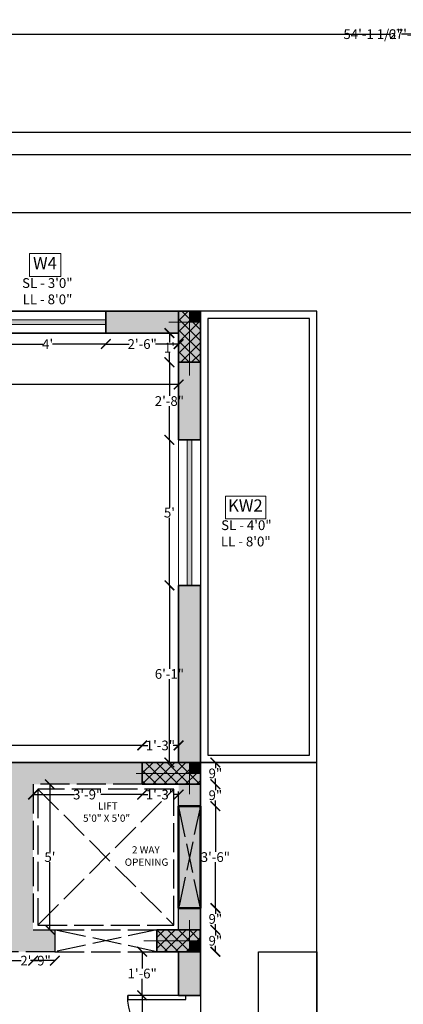
# Model space of a CAD drawing. Units: inches. Extents: x 2 to 905, y 9 to 678.
# Tile 6 of 8: x 295 to 454, y 272 to 678. Entities that reach past the tile are written whole.
import ezdxf

# ---------------------------------------------------------------- set-up
doc = ezdxf.new("R2010")
doc.units = ezdxf.units.IN
doc.linetypes.add('ACAD_ISO02W100', pattern=[15, 12, -3])
for name, color, linetype, lineweight in [('A-ANNO-DIMS', 7, 'Continuous', 18), ('A-COLS', 1, 'Continuous', 35), ('A-COLS-MARK', 1, 'Continuous', 18), ('A-COLS-MARK-PATT', 3, 'Continuous', 13), ('A-COLS-PATT', 1, 'Continuous', 13), ('A-DOOR', 7, 'Continuous', 25), ('A-FLOR', 7, 'Continuous', 25), ('A-GLAZ', 4, 'Continuous', 18), ('A-GLAZ-PATT', 4, 'Continuous', 13), ('A-TRAN', 1, 'Continuous', 50), ('A-TRAN-HIDN', 7, 'ACAD_ISO02W100', 25), ('A-WALL', 7, 'Continuous', 35), ('C-PROP', 7, 'Continuous', 25)]:
    doc.layers.add(name, color=color, linetype=linetype, lineweight=lineweight)
for name, color, linetype, lineweight, true_color in [('A-ANNO-IDEN', 251, 'Continuous', 18, 0x636466), ('A-ANNO-TEXT', 251, 'Continuous', 18, 0x636466), ('A-AREA-IDEN', 252, 'Continuous', 18, 0x989898), ('A-WALL-PATT', 252, 'Continuous', 13, 0x939598)]:
    doc.layers.add(name, color=color, linetype=linetype, lineweight=lineweight, true_color=true_color)
doc.styles.add('PDF ArialMT', font='arial.ttf')
doc.styles.add('PDF Century Gothic Bold', font='txt')
doc.styles.get("Standard").update_dxf_attribs({"font": 'arial.ttf'})
doc.dimstyles.get("Standard").update_dxf_attribs({"dimtxt": 4, "dimasz": 4, "dimexe": 0.18, "dimexo": 0.0625, "dimgap": 0.09, "dimtad": 0, "dimtih": 1, "dimtoh": 1, "dimdec": 1, "dimzin": 0, "dimdsep": 46, "dimlunit": 3, "dimtxsty": 'Standard', "dimblk": 'ARCHTICK', "dimcen": 0, "dimse1": 1, "dimse2": 1, "dimclrt": 1, "dimadec": 0, "dimazin": 0, "dimtfac": 1, "dimtdec": 1, "dimtofl": 0, "dimtmove": 0, "dimatfit": 3, "dimfxl": 1, "dimtolj": 1, "dimtzin": 0, "dimarcsym": 0})

# ---------------------------------------------------------------- blocks, each defined once
blk = doc.blocks.new('*U2')
for p, q in [((0, 0), (0, -6)), ((24, 0), (24, -6))]:
    blk.add_line(p, q)
blk.add_lwpolyline([(0, 0), (0, 24), (1.75, 24), (1.75, 0)], close=True)
blk.add_arc((0, 0), 24, 0, 90)
blk = doc.blocks.new('_ArchTick')
at = {"color": 0, "linetype": 'ByBlock', "const_width": 0.15}
blk.add_lwpolyline([(-0.5, -0.5), (0.5, 0.5)], dxfattribs=at)
blk = doc.blocks.new('*D11')
at = {"layer": 'A-ANNO-DIMS', "color": 0, "lineweight": -2, "transparency": 16777216}
for p, q in [((218.07, 548.58), (218.07, 462.21)), ((218.07, 371.58), (218.07, 457.95))]:
    blk.add_line(p, q, dxfattribs=at)
at = {"layer": 'Defpoints', "color": 0, "transparency": 16777216}
for p in [(360.93, 548.58), (218.07, 371.58), (360.93, 371.58)]:
    blk.add_point(p, dxfattribs=at)
at = {"layer": 'A-ANNO-DIMS', "color": 0, "lineweight": -2, "transparency": 16777216, "xscale": 4, "yscale": 4, "zscale": 4}
for p, rotation in [((218.07, 548.58), 90), ((218.07, 371.58), 270)]:
    blk.add_blockref('_ArchTick', p, dxfattribs=dict(at, rotation=rotation))
at = {"layer": 'A-ANNO-DIMS', "color": 0, "transparency": 16777216, "insert": (218.07, 460.08), "char_height": 4, "attachment_point": 5}
blk.add_mtext('\\A1;14\'-9"', dxfattribs=at)
blk = doc.blocks.new('*D12')
at = {"layer": 'A-ANNO-DIMS', "color": 0, "lineweight": -2, "transparency": 16777216}
for p, q in [((125.43, 527.38), (234.08, 527.38)), ((360.93, 527.38), (252.29, 527.38))]:
    blk.add_line(p, q, dxfattribs=at)
at = {"layer": 'Defpoints', "color": 0, "transparency": 16777216}
for p in [(125.43, 548.58), (360.93, 548.58), (360.93, 527.38)]:
    blk.add_point(p, dxfattribs=at)
at = {"layer": 'A-ANNO-DIMS', "color": 0, "lineweight": -2, "transparency": 16777216, "xscale": 4, "yscale": 4, "zscale": 4, "rotation": 180}
blk.add_blockref('_ArchTick', (125.43, 527.38), dxfattribs=at)
at = {"layer": 'A-ANNO-DIMS', "color": 0, "lineweight": -2, "transparency": 16777216, "xscale": 4, "yscale": 4, "zscale": 4}
blk.add_blockref('_ArchTick', (360.93, 527.38), dxfattribs=at)
at = {"layer": 'A-ANNO-DIMS', "color": 0, "transparency": 16777216, "insert": (243.18, 527.38), "char_height": 4, "attachment_point": 5}
blk.add_mtext('\\A1;19\'-7.5"', dxfattribs=at)
blk = doc.blocks.new('*D21')
at = {"layer": 'A-ANNO-DIMS', "color": 0, "lineweight": -2, "transparency": 16777216}
for p, q in [((345.92, 275.58), (345.92, 253.67)), ((345.92, 227.58), (345.92, 249.49))]:
    blk.add_line(p, q, dxfattribs=at)
at = {"layer": 'Defpoints', "color": 0, "transparency": 16777216}
for p in [(345.92, 275.58), (360.93, 275.58), (351.93, 227.58)]:
    blk.add_point(p, dxfattribs=at)
at = {"layer": 'A-ANNO-DIMS', "color": 0, "lineweight": -2, "transparency": 16777216, "xscale": 4, "yscale": 4, "zscale": 4}
for p, rotation in [((345.92, 275.58), 90), ((345.92, 227.58), 270)]:
    blk.add_blockref('_ArchTick', p, dxfattribs=dict(at, rotation=rotation))
at = {"layer": 'A-ANNO-DIMS', "color": 0, "transparency": 16777216, "insert": (345.92, 251.58), "char_height": 4, "attachment_point": 5}
blk.add_mtext("\\A1;4'", dxfattribs=at)
blk = doc.blocks.new('*D22')
at = {"layer": 'A-ANNO-DIMS', "color": 0, "lineweight": -2, "transparency": 16777216}
for p, q in [((345.92, 293.58), (345.92, 286.71)), ((345.92, 275.58), (345.92, 282.45))]:
    blk.add_line(p, q, dxfattribs=at)
at = {"layer": 'Defpoints', "color": 0, "transparency": 16777216}
for p in [(345.92, 293.58), (360.93, 293.58), (360.93, 275.58)]:
    blk.add_point(p, dxfattribs=at)
at = {"layer": 'A-ANNO-DIMS', "color": 0, "lineweight": -2, "transparency": 16777216, "xscale": 4, "yscale": 4, "zscale": 4}
for p, rotation in [((345.92, 293.58), 90), ((345.92, 275.58), 270)]:
    blk.add_blockref('_ArchTick', p, dxfattribs=dict(at, rotation=rotation))
at = {"layer": 'A-ANNO-DIMS', "color": 0, "transparency": 16777216, "insert": (345.92, 284.58), "char_height": 4, "attachment_point": 5}
blk.add_mtext('\\A1;1\'-6"', dxfattribs=at)
blk = doc.blocks.new('*D30')
at = {"layer": 'A-ANNO-DIMS', "color": 0, "lineweight": -2, "transparency": 16777216}
for p, q in [((285.93, 289.89), (295.97, 289.89)), ((309.93, 289.89), (299.9, 289.89))]:
    blk.add_line(p, q, dxfattribs=at)
at = {"layer": 'Defpoints', "color": 0, "transparency": 16777216}
for p in [(285.93, 293.58), (309.93, 293.58), (309.93, 289.89)]:
    blk.add_point(p, dxfattribs=at)
at = {"layer": 'A-ANNO-DIMS', "color": 0, "lineweight": -2, "transparency": 16777216, "xscale": 4, "yscale": 4, "zscale": 4, "rotation": 180}
blk.add_blockref('_ArchTick', (285.93, 289.89), dxfattribs=at)
at = {"layer": 'A-ANNO-DIMS', "color": 0, "lineweight": -2, "transparency": 16777216, "xscale": 4, "yscale": 4, "zscale": 4}
blk.add_blockref('_ArchTick', (309.93, 289.89), dxfattribs=at)
at = {"layer": 'A-ANNO-DIMS', "color": 0, "transparency": 16777216, "insert": (297.93, 289.89), "char_height": 4, "attachment_point": 5}
blk.add_mtext("\\A1;2'", dxfattribs=at)
blk = doc.blocks.new('*D31')
at = {"layer": 'A-ANNO-DIMS', "color": 0, "lineweight": -2, "transparency": 16777216}
for p, q in [((300.93, 289.89), (303.04, 289.89)), ((309.93, 289.89), (307.82, 289.89))]:
    blk.add_line(p, q, dxfattribs=at)
at = {"layer": 'Defpoints', "color": 0, "transparency": 16777216}
for p in [(300.93, 302.58), (309.93, 293.58), (300.93, 289.89)]:
    blk.add_point(p, dxfattribs=at)
at = {"layer": 'A-ANNO-DIMS', "color": 0, "lineweight": -2, "transparency": 16777216, "xscale": 4, "yscale": 4, "zscale": 4, "rotation": 180}
blk.add_blockref('_ArchTick', (300.93, 289.89), dxfattribs=at)
at = {"layer": 'A-ANNO-DIMS', "color": 0, "lineweight": -2, "transparency": 16777216, "xscale": 4, "yscale": 4, "zscale": 4}
blk.add_blockref('_ArchTick', (309.93, 289.89), dxfattribs=at)
at = {"layer": 'A-ANNO-DIMS', "color": 0, "transparency": 16777216, "insert": (305.43, 289.89), "char_height": 4, "attachment_point": 5}
blk.add_mtext('\\A1;9"', dxfattribs=at)
blk = doc.blocks.new('*D41')
at = {"layer": 'A-ANNO-DIMS', "color": 0, "lineweight": -2, "transparency": 16777216}
for p, q in [((300.93, 358.35), (318.03, 358.35)), ((345.93, 358.35), (328.84, 358.35))]:
    blk.add_line(p, q, dxfattribs=at)
at = {"layer": 'Defpoints', "color": 0, "transparency": 16777216}
for p in [(300.93, 362.58), (345.93, 362.58), (345.93, 358.35)]:
    blk.add_point(p, dxfattribs=at)
at = {"layer": 'A-ANNO-DIMS', "color": 0, "lineweight": -2, "transparency": 16777216, "xscale": 4, "yscale": 4, "zscale": 4, "rotation": 180}
blk.add_blockref('_ArchTick', (300.93, 358.35), dxfattribs=at)
at = {"layer": 'A-ANNO-DIMS', "color": 0, "lineweight": -2, "transparency": 16777216, "xscale": 4, "yscale": 4, "zscale": 4}
blk.add_blockref('_ArchTick', (345.93, 358.35), dxfattribs=at)
at = {"layer": 'A-ANNO-DIMS', "color": 0, "transparency": 16777216, "insert": (323.43, 358.35), "char_height": 4, "attachment_point": 5}
blk.add_mtext('\\A1;3\'-9"', dxfattribs=at)
blk = doc.blocks.new('*D42')
at = {"layer": 'A-ANNO-DIMS', "color": 0, "lineweight": -2, "transparency": 16777216}
for p, q in [((345.93, 358.35), (348.22, 358.35)), ((360.93, 358.35), (358.65, 358.35))]:
    blk.add_line(p, q, dxfattribs=at)
at = {"layer": 'Defpoints', "color": 0, "transparency": 16777216}
for p in [(345.93, 362.58), (360.93, 362.58), (360.93, 358.35)]:
    blk.add_point(p, dxfattribs=at)
at = {"layer": 'A-ANNO-DIMS', "color": 0, "lineweight": -2, "transparency": 16777216, "xscale": 4, "yscale": 4, "zscale": 4, "rotation": 180}
blk.add_blockref('_ArchTick', (345.93, 358.35), dxfattribs=at)
at = {"layer": 'A-ANNO-DIMS', "color": 0, "lineweight": -2, "transparency": 16777216, "xscale": 4, "yscale": 4, "zscale": 4}
blk.add_blockref('_ArchTick', (360.93, 358.35), dxfattribs=at)
at = {"layer": 'A-ANNO-DIMS', "color": 0, "transparency": 16777216, "insert": (353.43, 358.35), "char_height": 4, "attachment_point": 5}
blk.add_mtext('\\A1;1\'-3"', dxfattribs=at)
blk = doc.blocks.new('*D43')
at = {"layer": 'A-ANNO-DIMS', "color": 0, "lineweight": -2, "transparency": 16777216}
for p, q in [((307.87, 362.58), (307.87, 334.7)), ((307.87, 302.58), (307.87, 330.45))]:
    blk.add_line(p, q, dxfattribs=at)
at = {"layer": 'Defpoints', "color": 0, "transparency": 16777216}
for p in [(300.93, 362.58), (300.93, 302.58), (307.87, 302.58)]:
    blk.add_point(p, dxfattribs=at)
at = {"layer": 'A-ANNO-DIMS', "color": 0, "lineweight": -2, "transparency": 16777216, "xscale": 4, "yscale": 4, "zscale": 4}
for p, rotation in [((307.87, 362.58), 90), ((307.87, 302.58), 270)]:
    blk.add_blockref('_ArchTick', p, dxfattribs=dict(at, rotation=rotation))
at = {"layer": 'A-ANNO-DIMS', "color": 0, "transparency": 16777216, "insert": (307.87, 332.58), "char_height": 4, "attachment_point": 5}
blk.add_mtext("\\A1;5'", dxfattribs=at)
blk = doc.blocks.new('*D58')
at = {"layer": 'A-ANNO-DIMS', "color": 0, "lineweight": -2, "transparency": 16777216}
for p, q in [((282.93, 544.07), (304.92, 544.07)), ((330.93, 544.07), (308.94, 544.07))]:
    blk.add_line(p, q, dxfattribs=at)
at = {"layer": 'Defpoints', "color": 0, "transparency": 16777216}
for p in [(282.93, 548.58), (330.93, 548.58), (330.93, 544.07)]:
    blk.add_point(p, dxfattribs=at)
at = {"layer": 'A-ANNO-DIMS', "color": 0, "lineweight": -2, "transparency": 16777216, "xscale": 4, "yscale": 4, "zscale": 4, "rotation": 180}
blk.add_blockref('_ArchTick', (282.93, 544.07), dxfattribs=at)
at = {"layer": 'A-ANNO-DIMS', "color": 0, "lineweight": -2, "transparency": 16777216, "xscale": 4, "yscale": 4, "zscale": 4}
blk.add_blockref('_ArchTick', (330.93, 544.07), dxfattribs=at)
at = {"layer": 'A-ANNO-DIMS', "color": 0, "transparency": 16777216, "insert": (306.93, 544.07), "char_height": 4, "attachment_point": 5}
blk.add_mtext("\\A1;4'", dxfattribs=at)
blk = doc.blocks.new('*D59')
at = {"layer": 'A-ANNO-DIMS', "color": 0, "lineweight": -2, "transparency": 16777216}
for p, q in [((330.93, 544.07), (340.49, 544.07)), ((360.93, 544.07), (351.37, 544.07))]:
    blk.add_line(p, q, dxfattribs=at)
at = {"layer": 'Defpoints', "color": 0, "transparency": 16777216}
for p in [(330.93, 548.58), (360.93, 547.08), (360.93, 544.07)]:
    blk.add_point(p, dxfattribs=at)
at = {"layer": 'A-ANNO-DIMS', "color": 0, "lineweight": -2, "transparency": 16777216, "xscale": 4, "yscale": 4, "zscale": 4, "rotation": 180}
blk.add_blockref('_ArchTick', (330.93, 544.07), dxfattribs=at)
at = {"layer": 'A-ANNO-DIMS', "color": 0, "lineweight": -2, "transparency": 16777216, "xscale": 4, "yscale": 4, "zscale": 4}
blk.add_blockref('_ArchTick', (360.93, 544.07), dxfattribs=at)
at = {"layer": 'A-ANNO-DIMS', "color": 0, "transparency": 16777216, "insert": (345.93, 544.07), "char_height": 4, "attachment_point": 5}
blk.add_mtext('\\A1;2\'-6"', dxfattribs=at)
blk = doc.blocks.new('*D60')
at = {"layer": 'A-ANNO-DIMS', "color": 0, "lineweight": -2, "transparency": 16777216}
for p, q in [((357.15, 548.58), (357.15, 544.68)), ((357.15, 536.58), (357.15, 540.48))]:
    blk.add_line(p, q, dxfattribs=at)
at = {"layer": 'Defpoints', "color": 0, "transparency": 16777216}
for p in [(360.93, 548.58), (357.15, 536.58), (360.93, 536.58)]:
    blk.add_point(p, dxfattribs=at)
at = {"layer": 'A-ANNO-DIMS', "color": 0, "lineweight": -2, "transparency": 16777216, "xscale": 4, "yscale": 4, "zscale": 4}
for p, rotation in [((357.15, 548.58), 90), ((357.15, 536.58), 270)]:
    blk.add_blockref('_ArchTick', p, dxfattribs=dict(at, rotation=rotation))
at = {"layer": 'A-ANNO-DIMS', "color": 0, "transparency": 16777216, "insert": (357.15, 542.58), "char_height": 4, "attachment_point": 5}
blk.add_mtext("\\A1;1'", dxfattribs=at)
blk = doc.blocks.new('*D61')
at = {"layer": 'A-ANNO-DIMS', "color": 0, "lineweight": -2, "transparency": 16777216}
for p, q in [((357.15, 536.58), (357.15, 522.71)), ((357.15, 504.58), (357.15, 518.45))]:
    blk.add_line(p, q, dxfattribs=at)
at = {"layer": 'Defpoints', "color": 0, "transparency": 16777216}
for p in [(360.93, 536.58), (357.15, 504.58), (360.93, 504.58)]:
    blk.add_point(p, dxfattribs=at)
at = {"layer": 'A-ANNO-DIMS', "color": 0, "lineweight": -2, "transparency": 16777216, "xscale": 4, "yscale": 4, "zscale": 4}
for p, rotation in [((357.15, 536.58), 90), ((357.15, 504.58), 270)]:
    blk.add_blockref('_ArchTick', p, dxfattribs=dict(at, rotation=rotation))
at = {"layer": 'A-ANNO-DIMS', "color": 0, "transparency": 16777216, "insert": (357.15, 520.58), "char_height": 4, "attachment_point": 5}
blk.add_mtext('\\A1;2\'-8"', dxfattribs=at)
blk = doc.blocks.new('*D62')
at = {"layer": 'A-ANNO-DIMS', "color": 0, "lineweight": -2, "transparency": 16777216}
for p, q in [((357.15, 504.58), (357.15, 476.7)), ((357.15, 444.58), (357.15, 472.45))]:
    blk.add_line(p, q, dxfattribs=at)
at = {"layer": 'Defpoints', "color": 0, "transparency": 16777216}
for p in [(360.93, 504.58), (357.15, 444.58), (360.93, 444.58)]:
    blk.add_point(p, dxfattribs=at)
at = {"layer": 'A-ANNO-DIMS', "color": 0, "lineweight": -2, "transparency": 16777216, "xscale": 4, "yscale": 4, "zscale": 4}
for p, rotation in [((357.15, 504.58), 90), ((357.15, 444.58), 270)]:
    blk.add_blockref('_ArchTick', p, dxfattribs=dict(at, rotation=rotation))
at = {"layer": 'A-ANNO-DIMS', "color": 0, "transparency": 16777216, "insert": (357.15, 474.58), "char_height": 4, "attachment_point": 5}
blk.add_mtext("\\A1;5'", dxfattribs=at)
blk = doc.blocks.new('*D63')
at = {"layer": 'A-ANNO-DIMS', "color": 0, "lineweight": -2, "transparency": 16777216}
for p, q in [((357.15, 444.58), (357.15, 410.21)), ((357.15, 371.58), (357.15, 405.95))]:
    blk.add_line(p, q, dxfattribs=at)
at = {"layer": 'Defpoints', "color": 0, "transparency": 16777216}
for p in [(360.93, 444.58), (357.15, 371.58), (360.93, 371.58)]:
    blk.add_point(p, dxfattribs=at)
at = {"layer": 'A-ANNO-DIMS', "color": 0, "lineweight": -2, "transparency": 16777216, "xscale": 4, "yscale": 4, "zscale": 4}
for p, rotation in [((357.15, 444.58), 90), ((357.15, 371.58), 270)]:
    blk.add_blockref('_ArchTick', p, dxfattribs=dict(at, rotation=rotation))
at = {"layer": 'A-ANNO-DIMS', "color": 0, "transparency": 16777216, "insert": (357.15, 408.08), "char_height": 4, "attachment_point": 5}
blk.add_mtext('\\A1;6\'-1"', dxfattribs=at)
blk = doc.blocks.new('*D64')
at = {"layer": 'A-ANNO-DIMS', "color": 0, "lineweight": -2, "transparency": 16777216}
for p, q in [((345.93, 378.61), (348.22, 378.61)), ((360.93, 378.61), (358.65, 378.61))]:
    blk.add_line(p, q, dxfattribs=at)
at = {"layer": 'Defpoints', "color": 0, "transparency": 16777216}
for p in [(345.93, 378.61), (345.93, 371.58), (360.93, 371.58)]:
    blk.add_point(p, dxfattribs=at)
at = {"layer": 'A-ANNO-DIMS', "color": 0, "lineweight": -2, "transparency": 16777216, "xscale": 4, "yscale": 4, "zscale": 4, "rotation": 180}
blk.add_blockref('_ArchTick', (345.93, 378.61), dxfattribs=at)
at = {"layer": 'A-ANNO-DIMS', "color": 0, "lineweight": -2, "transparency": 16777216, "xscale": 4, "yscale": 4, "zscale": 4}
blk.add_blockref('_ArchTick', (360.93, 378.61), dxfattribs=at)
at = {"layer": 'A-ANNO-DIMS', "color": 0, "transparency": 16777216, "insert": (353.43, 378.61), "char_height": 4, "attachment_point": 5}
blk.add_mtext('\\A1;1\'-3"', dxfattribs=at)
blk = doc.blocks.new('*D65')
at = {"layer": 'A-ANNO-DIMS', "color": 0, "lineweight": -2, "transparency": 16777216}
for p, q in [((183.93, 378.61), (258.16, 378.61)), ((345.93, 378.61), (271.71, 378.61))]:
    blk.add_line(p, q, dxfattribs=at)
at = {"layer": 'Defpoints', "color": 0, "transparency": 16777216}
for p in [(183.93, 378.61), (183.93, 371.58), (345.93, 371.58)]:
    blk.add_point(p, dxfattribs=at)
at = {"layer": 'A-ANNO-DIMS', "color": 0, "lineweight": -2, "transparency": 16777216, "xscale": 4, "yscale": 4, "zscale": 4, "rotation": 180}
blk.add_blockref('_ArchTick', (183.93, 378.61), dxfattribs=at)
at = {"layer": 'A-ANNO-DIMS', "color": 0, "lineweight": -2, "transparency": 16777216, "xscale": 4, "yscale": 4, "zscale": 4}
blk.add_blockref('_ArchTick', (345.93, 378.61), dxfattribs=at)
at = {"layer": 'A-ANNO-DIMS', "color": 0, "transparency": 16777216, "insert": (264.93, 378.61), "char_height": 4, "attachment_point": 5}
blk.add_mtext('\\A1;13\'-6"', dxfattribs=at)
blk = doc.blocks.new('*D85')
at = {"layer": 'A-ANNO-DIMS', "color": 0, "lineweight": -2, "transparency": 16777216}
for p, q in [((376.1, 302.58), (376.1, 300.21)), ((376.1, 293.58), (376.1, 295.95))]:
    blk.add_line(p, q, dxfattribs=at)
at = {"layer": 'Defpoints', "color": 0, "transparency": 16777216}
for p in [(369.88, 302.58), (376.1, 302.58), (369.88, 293.58)]:
    blk.add_point(p, dxfattribs=at)
at = {"layer": 'A-ANNO-DIMS', "color": 0, "lineweight": -2, "transparency": 16777216, "xscale": 4, "yscale": 4, "zscale": 4}
for p, rotation in [((376.1, 302.58), 90), ((376.1, 293.58), 270)]:
    blk.add_blockref('_ArchTick', p, dxfattribs=dict(at, rotation=rotation))
at = {"layer": 'A-ANNO-DIMS', "color": 0, "transparency": 16777216, "insert": (376.1, 298.08), "char_height": 4, "attachment_point": 5}
blk.add_mtext('\\A1;9"', dxfattribs=at)
blk = doc.blocks.new('*D86')
at = {"layer": 'A-ANNO-DIMS', "color": 0, "lineweight": -2, "transparency": 16777216}
for p, q in [((376.1, 311.58), (376.1, 309.21)), ((376.1, 302.58), (376.1, 304.95))]:
    blk.add_line(p, q, dxfattribs=at)
at = {"layer": 'Defpoints', "color": 0, "transparency": 16777216}
for p in [(369.93, 311.58), (376.1, 311.58), (369.88, 302.58)]:
    blk.add_point(p, dxfattribs=at)
at = {"layer": 'A-ANNO-DIMS', "color": 0, "lineweight": -2, "transparency": 16777216, "xscale": 4, "yscale": 4, "zscale": 4}
for p, rotation in [((376.1, 311.58), 90), ((376.1, 302.58), 270)]:
    blk.add_blockref('_ArchTick', p, dxfattribs=dict(at, rotation=rotation))
at = {"layer": 'A-ANNO-DIMS', "color": 0, "transparency": 16777216, "insert": (376.1, 307.08), "char_height": 4, "attachment_point": 5}
blk.add_mtext('\\A1;9"', dxfattribs=at)
blk = doc.blocks.new('*D87')
at = {"layer": 'A-ANNO-DIMS', "color": 0, "lineweight": -2, "transparency": 16777216}
for p, q in [((376.1, 353.58), (376.1, 334.71)), ((376.1, 311.58), (376.1, 330.44))]:
    blk.add_line(p, q, dxfattribs=at)
at = {"layer": 'Defpoints', "color": 0, "transparency": 16777216}
for p in [(369.93, 353.58), (376.1, 353.58), (369.93, 311.58)]:
    blk.add_point(p, dxfattribs=at)
at = {"layer": 'A-ANNO-DIMS', "color": 0, "lineweight": -2, "transparency": 16777216, "xscale": 4, "yscale": 4, "zscale": 4}
for p, rotation in [((376.1, 353.58), 90), ((376.1, 311.58), 270)]:
    blk.add_blockref('_ArchTick', p, dxfattribs=dict(at, rotation=rotation))
at = {"layer": 'A-ANNO-DIMS', "color": 0, "transparency": 16777216, "insert": (376.1, 332.58), "char_height": 4, "attachment_point": 5}
blk.add_mtext('\\A1;3\'-6"', dxfattribs=at)
blk = doc.blocks.new('*D88')
at = {"layer": 'A-ANNO-DIMS', "color": 0, "lineweight": -2, "transparency": 16777216}
for p, q in [((376.1, 362.58), (376.1, 360.21)), ((376.1, 353.58), (376.1, 355.95))]:
    blk.add_line(p, q, dxfattribs=at)
at = {"layer": 'Defpoints', "color": 0, "transparency": 16777216}
for p in [(369.93, 362.58), (376.1, 362.58), (369.93, 353.58)]:
    blk.add_point(p, dxfattribs=at)
at = {"layer": 'A-ANNO-DIMS', "color": 0, "lineweight": -2, "transparency": 16777216, "xscale": 4, "yscale": 4, "zscale": 4}
for p, rotation in [((376.1, 362.58), 90), ((376.1, 353.58), 270)]:
    blk.add_blockref('_ArchTick', p, dxfattribs=dict(at, rotation=rotation))
at = {"layer": 'A-ANNO-DIMS', "color": 0, "transparency": 16777216, "insert": (376.1, 358.08), "char_height": 4, "attachment_point": 5}
blk.add_mtext('\\A1;9"', dxfattribs=at)
blk = doc.blocks.new('*D89')
at = {"layer": 'A-ANNO-DIMS', "color": 0, "lineweight": -2, "transparency": 16777216}
for p, q in [((376.1, 371.58), (376.1, 369.21)), ((376.1, 362.58), (376.1, 364.95))]:
    blk.add_line(p, q, dxfattribs=at)
at = {"layer": 'Defpoints', "color": 0, "transparency": 16777216}
for p in [(369.93, 371.58), (376.1, 371.58), (369.93, 362.58)]:
    blk.add_point(p, dxfattribs=at)
at = {"layer": 'A-ANNO-DIMS', "color": 0, "lineweight": -2, "transparency": 16777216, "xscale": 4, "yscale": 4, "zscale": 4}
for p, rotation in [((376.1, 371.58), 90), ((376.1, 362.58), 270)]:
    blk.add_blockref('_ArchTick', p, dxfattribs=dict(at, rotation=rotation))
at = {"layer": 'A-ANNO-DIMS', "color": 0, "transparency": 16777216, "insert": (376.1, 367.08), "char_height": 4, "attachment_point": 5}
blk.add_mtext('\\A1;9"', dxfattribs=at)
blk = doc.blocks.new('COL-DATUM-R')
h = blk.add_hatch(color=256)
h.dxf.hatch_style = 1
h.paths.add_polyline_path([(13.01, 0), (13.01, 4.5), (8.51, 4.5), (8.51, 0)])
for p, q in [((8.51, 0), (8.51, 26.48)), ((13.01, 4.5), (0, 4.5))]:
    blk.add_line(p, q)
blk.add_lwpolyline([(8.51, 0), (13.01, 0), (13.01, 4.5), (8.51, 4.5)], close=True)
blk = doc.blocks.new('COL-DATUM-L')
h = blk.add_hatch(color=256)
h.dxf.hatch_style = 1
h.paths.add_polyline_path([(4.5, 0), (4.5, 4.5), (0, 4.5), (0, 0)])
for p, q in [((4.5, 0), (4.5, 26.48)), ((0, 4.5), (13.01, 4.5))]:
    blk.add_line(p, q)
blk.add_lwpolyline([(4.5, 0), (0, 0), (0, 4.5), (4.5, 4.5)], close=True)
blk = doc.blocks.new('GLAZ-W4-48')
h = blk.add_hatch(color=256)
h.dxf.hatch_style = 1
h.paths.add_polyline_path([(48, 0), (48, 2), (0, 2), (0, 0)])
for p, q in [((0, 2), (48, 2)), ((0, 0), (48, 0))]:
    blk.add_line(p, q)
blk = doc.blocks.new('COL-DATUM-CROSS-SHORT')
for p, q in [((18.83, 0), (18.83, 13.01)), ((23.33, 4.5), (0, 4.5))]:
    blk.add_line(p, q)
blk = doc.blocks.new('*D102')
at = {"layer": 'A-ANNO-DIMS', "color": 0, "lineweight": -2, "transparency": 16777216}
for p, q in [((53.05, 671.82), (448.08, 671.82)), ((857.05, 671.82), (462.03, 671.82))]:
    blk.add_line(p, q, dxfattribs=at)
at = {"layer": 'Defpoints', "color": 0, "transparency": 16777216}
for p in [(857.05, 671.82), (53.05, 631.22), (857.05, 631.22)]:
    blk.add_point(p, dxfattribs=at)
at = {"layer": 'A-ANNO-DIMS', "color": 0, "lineweight": -2, "transparency": 16777216, "xscale": 4, "yscale": 4, "zscale": 4, "rotation": 180}
blk.add_blockref('_ArchTick', (53.05, 671.82), dxfattribs=at)
at = {"layer": 'A-ANNO-DIMS', "color": 0, "lineweight": -2, "transparency": 16777216, "xscale": 4, "yscale": 4, "zscale": 4}
blk.add_blockref('_ArchTick', (857.05, 671.82), dxfattribs=at)
at = {"layer": 'A-ANNO-DIMS', "color": 1, "transparency": 16777216, "insert": (455.05, 671.82), "char_height": 4, "attachment_point": 5}
blk.add_mtext('\\A1;67\'-0"', dxfattribs=at)
blk = doc.blocks.new('*D108')
at = {"layer": 'A-ANNO-DIMS', "color": 0, "lineweight": -2, "transparency": 16777216}
for p, q in [((897.65, 622.22), (897.65, 612.35)), ((897.65, 598.22), (897.65, 608.09))]:
    blk.add_line(p, q, dxfattribs=at)
at = {"layer": 'Defpoints', "color": 0, "transparency": 16777216}
for p in [(62.05, 622.22), (86.05, 598.22), (897.65, 598.22)]:
    blk.add_point(p, dxfattribs=at)
at = {"layer": 'A-ANNO-DIMS', "color": 0, "lineweight": -2, "transparency": 16777216, "xscale": 4, "yscale": 4, "zscale": 4}
for p, rotation in [((897.65, 622.22), 90), ((897.65, 598.22), 270)]:
    blk.add_blockref('_ArchTick', p, dxfattribs=dict(at, rotation=rotation))
at = {"layer": 'A-ANNO-DIMS', "color": 1, "transparency": 16777216, "insert": (897.65, 610.22), "char_height": 4, "attachment_point": 5}
blk.add_mtext('\\A1;2\'-0"', dxfattribs=at)
blk = doc.blocks.new('*D111')
at = {"layer": 'A-ANNO-DIMS', "color": 0, "lineweight": -2, "transparency": 16777216}
for p, q in [((116.43, 671.82), (429.56, 671.82)), ((765.93, 671.82), (452.8, 671.82))]:
    blk.add_line(p, q, dxfattribs=at)
at = {"layer": 'Defpoints', "color": 0, "transparency": 16777216}
for p in [(765.93, 671.82), (116.43, 557.58), (765.93, 557.58)]:
    blk.add_point(p, dxfattribs=at)
at = {"layer": 'A-ANNO-DIMS', "color": 0, "lineweight": -2, "transparency": 16777216, "xscale": 4, "yscale": 4, "zscale": 4, "rotation": 180}
blk.add_blockref('_ArchTick', (116.43, 671.82), dxfattribs=at)
at = {"layer": 'A-ANNO-DIMS', "color": 0, "lineweight": -2, "transparency": 16777216, "xscale": 4, "yscale": 4, "zscale": 4}
blk.add_blockref('_ArchTick', (765.93, 671.82), dxfattribs=at)
at = {"layer": 'A-ANNO-DIMS', "color": 1, "transparency": 16777216, "insert": (441.18, 671.82), "char_height": 4, "attachment_point": 5}
blk.add_mtext('\\A1;54\'-1 1/2"', dxfattribs=at)
blk = doc.blocks.new('*D112')
at = {"layer": 'A-ANNO-DIMS', "color": 0, "lineweight": -2, "transparency": 16777216}
for p, q in [((897.65, 557.58), (897.65, 345.21)), ((897.65, 128.58), (897.65, 340.94))]:
    blk.add_line(p, q, dxfattribs=at)
at = {"layer": 'Defpoints', "color": 0, "transparency": 16777216}
for p in [(417.93, 557.58), (897.65, 557.58), (417.93, 128.58)]:
    blk.add_point(p, dxfattribs=at)
at = {"layer": 'A-ANNO-DIMS', "color": 0, "lineweight": -2, "transparency": 16777216, "xscale": 4, "yscale": 4, "zscale": 4}
for p, rotation in [((897.65, 557.58), 90), ((897.65, 128.58), 270)]:
    blk.add_blockref('_ArchTick', p, dxfattribs=dict(at, rotation=rotation))
at = {"layer": 'A-ANNO-DIMS', "color": 1, "transparency": 16777216, "insert": (897.65, 343.08), "char_height": 4, "attachment_point": 5}
blk.add_mtext('\\A1;35\'-9"', dxfattribs=at)

msp = doc.modelspace()

# ---------------------------------------------------------------- hatches: boundary and pattern name
at = {"layer": 'A-COLS-MARK-PATT'}
h = msp.add_hatch(color=256, dxfattribs=at)
h.dxf.hatch_style = 1
h.paths.add_polyline_path([(369.88, 298.08), (365.38, 298.08), (365.38, 293.58), (369.88, 293.58)])
at = {"layer": 'A-COLS-PATT'}
h = msp.add_hatch(dxfattribs=at)
h.set_pattern_fill('ANSI37', color=256, angle=-180)
h.set_pattern_definition([(225, (-408.7418, 893.045), (2.245064, -2.245064), []), (315, (-408.7418, 893.045), (2.245064, 2.245064), [])])
h.paths.add_polyline_path([(360.93, 553.08), (365.43, 553.08), (365.43, 557.58), (360.93, 557.58)])
h.paths.add_polyline_path([(360.93, 536.58), (365.43, 536.58), (365.43, 553.08), (360.93, 553.08)])
h.paths.add_polyline_path([(365.43, 536.58), (369.93, 536.58), (369.93, 553.08), (365.43, 553.08)])
h = msp.add_hatch(dxfattribs=at)
h.set_pattern_fill('ANSI37', color=256, angle=90)
h.set_pattern_definition([(135, (546.4012, 949.2528), (-2.245064, -2.245064), []), (225, (546.4012, 949.2528), (2.245064, -2.245064), [])])
h.paths.add_polyline_path([(365.43, 362.58), (365.43, 367.08), (369.93, 367.08), (369.93, 362.58)])
h.paths.add_polyline_path([(345.93, 362.58), (345.93, 367.08), (365.43, 367.08), (365.43, 362.58)])
h.paths.add_polyline_path([(345.93, 367.08), (345.93, 371.58), (365.43, 371.58), (365.43, 367.08)])
h = msp.add_hatch(dxfattribs=at)
h.set_pattern_fill('ANSI37', color=256, angle=90)
h.set_pattern_definition([(135, (645.35, 871.2528), (-2.245064, -2.245064), []), (225, (645.35, 871.2528), (2.245064, -2.245064), [])])
h.paths.add_polyline_path([(365.38, 302.58), (365.38, 298.08), (369.88, 298.08), (369.88, 302.58)])
h.paths.add_polyline_path([(351.93, 293.58), (351.93, 298.08), (365.38, 298.08), (365.38, 293.58)])
h.paths.add_polyline_path([(351.93, 298.08), (351.93, 302.58), (365.38, 302.58), (365.38, 298.08)])
at = {"layer": 'A-GLAZ-PATT'}
h = msp.add_hatch(color=256, dxfattribs=at)
h.dxf.hatch_style = 1
h.paths.add_polyline_path([(366.43, 504.58), (364.43, 504.58), (364.43, 444.58), (366.43, 444.58)])
at = {"layer": 'A-WALL-PATT'}
h = msp.add_hatch(color=256, dxfattribs=at)
h.dxf.hatch_style = 1
h.paths.add_polyline_path([(125.43, 227.58), (116.43, 227.58), (116.43, 128.58), (237.93, 128.58), (237.93, 137.58), (125.43, 137.58)])
h.paths.add_polyline_path([(249.93, 302.58), (183.93, 302.58), (183.93, 320.58), (179.43, 320.58), (179.43, 302.58), (116.43, 302.58), (116.43, 275.58), (125.43, 275.58), (125.43, 293.58), (249.93, 293.58), (249.93, 297.58)], flags=0)
h.paths.add_polyline_path([(369.93, 137.58), (360.93, 137.58), (360.93, 218.58), (369.93, 218.58), (369.93, 227.58), (363.93, 227.58), (351.93, 227.58), (351.93, 137.58), (345.93, 137.58), (345.93, 128.58), (360.93, 128.58), (369.93, 128.58)])
h.paths.add_polyline_path([(297.93, 137.58), (285.93, 137.58), (285.93, 128.58), (297.93, 128.58)])
h.paths.add_polyline_path([(369.93, 444.58), (360.93, 444.58), (360.93, 371.58), (183.93, 371.58), (183.93, 460.08), (125.43, 460.08), (125.43, 466.08), (116.43, 466.08), (116.43, 449.58), (120.43, 449.58), (125.43, 449.58), (125.43, 455.58), (179.43, 455.58), (179.43, 371.58), (125.43, 371.58), (125.43, 389.58), (116.43, 389.58), (116.43, 362.58), (179.43, 362.58), (179.43, 344.58), (183.93, 344.58), (183.93, 362.58), (291.93, 362.58), (291.93, 302.58), (285.93, 302.58), (285.93, 293.58), (309.93, 293.58), (309.93, 302.58), (300.93, 302.58), (300.93, 362.58), (360.93, 362.58), (360.93, 302.58), (351.93, 302.58), (351.93, 293.58), (360.93, 293.58), (360.93, 275.58), (363.93, 275.58), (369.93, 275.58)])
h.paths.add_polyline_path([(282.93, 557.58), (116.43, 557.58), (116.43, 506.08), (120.43, 506.08), (125.43, 506.08), (125.43, 548.58), (282.93, 548.58)])
h.paths.add_polyline_path([(369.93, 557.58), (330.93, 557.58), (330.93, 548.58), (360.93, 548.58), (360.93, 504.58), (369.93, 504.58)])

# ---------------------------------------------------------------- linework, layer by layer
at = {"layer": 'A-ANNO-IDEN'}
for points in [[(299.45, 581.45), (312.35, 581.45), (312.35, 571.97), (299.45, 571.97)], [(380.32, 481.41), (396.97, 481.41), (396.97, 472.04), (380.32, 472.04)]]:
    msp.add_lwpolyline(points, close=True, dxfattribs=at)
at = {"layer": 'A-COLS'}
for points in [[(369.93, 536.58), (360.93, 536.58), (360.93, 557.58), (369.93, 557.58)], [(345.93, 371.58), (345.93, 362.58), (369.93, 362.58), (369.93, 371.58)], [(351.93, 293.58), (351.93, 302.58), (369.88, 302.58), (369.88, 293.58)]]:
    msp.add_lwpolyline(points, close=True, dxfattribs=at)
at = {"layer": 'A-COLS-MARK'}
msp.add_lwpolyline([(369.88, 298.08), (369.88, 293.58), (365.38, 293.58), (365.38, 298.08)], close=True, dxfattribs=at)
at = {"layer": 'A-FLOR'}
for points in [[(369.93, 371.58), (417.93, 371.58), (417.93, 557.58), (369.93, 557.58)], [(372.93, 374.58), (414.93, 374.58), (414.93, 554.58), (372.93, 554.58)], [(369.93, 224.58), (417.93, 224.58), (417.93, 371.58), (369.93, 371.58)], [(417.93, 227.58), (393.93, 227.58), (393.93, 293.58), (417.93, 293.58)]]:
    msp.add_lwpolyline(points, close=True, dxfattribs=at)
at = {"layer": 'A-GLAZ'}
for p, q in [((364.43, 444.58), (364.43, 504.58)), ((366.43, 444.58), (366.43, 504.58))]:
    msp.add_line(p, q, dxfattribs=at)
for points in [[(282.93, 557.58), (330.93, 557.58), (330.93, 548.58), (282.93, 548.58)], [(360.93, 444.58), (360.93, 504.58), (369.93, 504.58), (369.93, 444.58)]]:
    msp.add_lwpolyline(points, close=True, dxfattribs=at)
at = {"layer": 'A-TRAN'}
msp.add_lwpolyline([(360.93, 311.58), (369.93, 311.58), (369.93, 353.58), (360.93, 353.58)], close=True, dxfattribs=at)
at = {"layer": 'A-TRAN-HIDN'}
for p, q in [((302.93, 304.58), (358.93, 360.58)), ((302.93, 360.58), (358.93, 304.58))]:
    msp.add_line(p, q, dxfattribs=at)
msp.add_lwpolyline([(360.93, 302.58), (360.93, 362.58), (300.93, 362.58), (300.93, 302.58), (309.93, 302.58), (351.93, 302.58), (309.93, 293.58), (351.93, 293.58), (309.93, 302.58), (309.93, 293.58), (285.93, 293.58), (285.93, 302.58), (291.93, 302.58)], dxfattribs=at)
for points in [[(358.93, 360.58), (302.93, 360.58), (302.93, 304.58), (358.93, 304.58)], [(369.93, 353.58), (360.93, 311.58), (369.93, 311.58), (360.93, 353.58)]]:
    msp.add_lwpolyline(points, close=True, dxfattribs=at)
at = {"layer": 'A-WALL'}
for p, q in [((360.93, 444.58), (369.93, 444.58)), ((360.93, 444.58), (360.93, 371.58)), ((369.93, 444.58), (369.93, 275.58)), ((183.93, 371.58), (360.93, 371.58)), ((360.93, 293.58), (360.93, 275.58)), ((369.93, 275.58), (360.93, 275.58))]:
    msp.add_line(p, q, dxfattribs=at)
for points in [[(125.43, 506.08), (116.43, 506.08), (116.43, 557.58), (369.93, 557.58), (369.93, 504.58), (360.93, 504.58), (369.93, 504.58), (360.93, 504.58), (360.93, 548.58), (125.43, 548.58)], [(330.93, 557.58), (330.93, 548.58)]]:
    msp.add_lwpolyline(points, close=True, dxfattribs=at)
msp.add_lwpolyline([(360.88, 302.58), (369.88, 302.58), (369.88, 293.58)], dxfattribs=at)
at = {"layer": 'C-PROP'}
msp.add_lwpolyline([(857.05, 535.22), (857.05, 631.22), (53.05, 631.22), (53.05, 55.22), (857.05, 55.22), (857.05, 355.22), (848.05, 355.22), (848.05, 64.22), (62.05, 64.22), (62.05, 622.22), (848.05, 622.22), (848.05, 535.22)], close=True, dxfattribs=at)
msp.add_lwpolyline([(848.05, 598.22), (86.05, 598.22), (86.05, 88.22), (824.05, 88.22), (824.05, 355.22), (836.05, 355.22), (848.05, 355.22)], dxfattribs=at)

# ---------------------------------------------------------------- block references
at = {"layer": 'A-COLS-MARK'}
for name, p, rotation in [('COL-DATUM-L', (369.93, 557.58), 180), ('COL-DATUM-R', (369.93, 358.57), 90.00000000000017)]:
    msp.add_blockref(name, p, dxfattribs=dict(at, rotation=rotation))
msp.add_blockref('COL-DATUM-CROSS-SHORT', (346.55, 293.58), dxfattribs=at)
at = {"layer": 'A-DOOR', "xscale": -1, "rotation": 90}
msp.add_blockref('*U2', (363.93, 275.58), dxfattribs=at)
at = {"layer": 'A-GLAZ'}
msp.add_blockref('GLAZ-W4-48', (282.93, 552.08), dxfattribs=at)

# ---------------------------------------------------------------- texts
at = {"layer": 'A-ANNO-IDEN', "attachment_point": 4, "style": 'PDF ArialMT'}
for s, insert, char_height in [('W4', (300.9, 576.8), 5.029), ('SL - 3\'0"', (296.38, 568.7), 4.023), ('LL - 8\'0"', (296.6, 561.97), 4.023), ('KW2', (381.34, 476.87), 5.029), ('SL - 4\'0"', (378.47, 468.88), 4.023), ('LL - 8\'0"', (378.36, 462.15), 4.023)]:
    msp.add_mtext(s, dxfattribs=dict(at, insert=insert, char_height=char_height))
at = {"layer": 'A-ANNO-TEXT', "char_height": 3, "attachment_point": 4, "style": 'PDF Century Gothic Bold'}
for s, insert in [('2 WAY', (341.7, 335.17)), ('OPENING', (338.72, 330.1))]:
    msp.add_mtext(s, dxfattribs=dict(at, insert=insert))
at = {"layer": 'A-AREA-IDEN', "char_height": 3, "attachment_point": 4, "style": 'PDF Century Gothic Bold'}
for s, insert in [('LIFT', (327.69, 353.3)), ('5\'0" X 5\'0"', (321.52, 348.23))]:
    msp.add_mtext(s, dxfattribs=dict(at, insert=insert))

# ---------------------------------------------------------------- dimensions: what is measured, and where the dimension line sits
at = {"layer": 'A-ANNO-DIMS'}
for base, p1, p2, override, picture, middle in [((857.05, 671.82), (53.05, 631.22), (857.05, 631.22), {"dimdec": 1, "dimlfac": 1, "dimrnd": 0, "dimzin": 1, "dimdsep": 46, "dimlunit": 4, "dimfrac": 2}, '*D102', (455.05, 671.82)), ((765.93, 671.82), (116.43, 557.58), (765.93, 557.58), {"dimdec": 1, "dimlfac": 1, "dimrnd": 0, "dimzin": 1, "dimdsep": 46, "dimlunit": 4, "dimfrac": 2}, '*D111', (441.18, 671.82)), ((360.93, 527.38), (125.43, 548.58), (360.93, 548.58), {"dimclrd": 0, "dimclre": 0, "dimclrt": 0}, '*D12', (243.18, 527.38)), ((330.93, 544.07), (282.93, 548.58), (330.93, 548.58), {"dimclrd": 0, "dimclre": 0, "dimclrt": 0, "dimtmove": 1}, '*D58', (306.93, 544.07)), ((360.93, 544.07), (330.93, 548.58), (360.93, 547.08), {"dimdec": 0, "dimclrd": 0, "dimclre": 0, "dimclrt": 0, "dimtmove": 1}, '*D59', (345.93, 544.07)), ((183.93, 378.61), (345.93, 371.58), (183.93, 371.58), {"dimdec": 0, "dimclrd": 0, "dimclre": 0, "dimclrt": 0, "dimtmove": 1}, '*D65', (264.93, 378.61)), ((345.93, 378.61), (360.93, 371.58), (345.93, 371.58), {"dimdec": 0, "dimclrd": 0, "dimclre": 0, "dimclrt": 0}, '*D64', (353.43, 378.61)), ((345.93, 358.35), (300.93, 362.58), (345.93, 362.58), {"dimdec": 0, "dimclrd": 0, "dimclre": 0, "dimclrt": 0}, '*D41', (323.43, 358.35)), ((360.93, 358.35), (345.93, 362.58), (360.93, 362.58), {"dimdec": 0, "dimclrd": 0, "dimclre": 0, "dimclrt": 0, "dimtmove": 1}, '*D42', (353.43, 358.35)), ((300.93, 289.89), (309.93, 293.58), (300.93, 302.58), {"dimdec": 0, "dimclrd": 0, "dimclre": 0, "dimclrt": 0, "dimtmove": 1}, '*D31', (305.43, 289.89)), ((309.93, 289.89), (285.93, 293.58), (309.93, 293.58), {"dimclrd": 0, "dimclre": 0, "dimclrt": 0, "dimtmove": 1}, '*D30', (297.93, 289.89))]:
    dim = msp.add_linear_dim(base=base, p1=p1, p2=p2, dimstyle='Standard', override=override, dxfattribs=at)
    dim.commit()
    dim.dimension.update_dxf_attribs({"geometry": picture, "text_midpoint": middle})
for base, p1, p2, override, picture, middle in [((897.65, 598.22), (62.05, 622.22), (86.05, 598.22), {"dimdec": 1, "dimlfac": 1, "dimrnd": 0, "dimzin": 1, "dimdsep": 46, "dimlunit": 4, "dimfrac": 2}, '*D108', (897.65, 610.22)), ((897.65, 557.58), (417.93, 128.58), (417.93, 557.58), {"dimdec": 1, "dimlfac": 1, "dimrnd": 0, "dimzin": 1, "dimdsep": 46, "dimlunit": 4, "dimfrac": 2}, '*D112', (897.65, 343.08)), ((218.07, 371.58), (360.93, 548.58), (360.93, 371.58), {"dimdec": 0, "dimclrd": 0, "dimclre": 0, "dimclrt": 0}, '*D11', (218.07, 460.08)), ((357.15, 536.58), (360.93, 548.58), (360.93, 536.58), {"dimclrd": 0, "dimclre": 0, "dimclrt": 0}, '*D60', (357.15, 542.58)), ((357.15, 504.58), (360.93, 536.58), (360.93, 504.58), {"dimdec": 0, "dimclrd": 0, "dimclre": 0, "dimclrt": 0, "dimtmove": 1}, '*D61', (357.15, 520.58)), ((357.15, 444.58), (360.93, 504.58), (360.93, 444.58), {"dimclrd": 0, "dimclre": 0, "dimclrt": 0, "dimtmove": 1}, '*D62', (357.15, 474.58)), ((357.15, 371.58), (360.93, 444.58), (360.93, 371.58), {"dimdec": 0, "dimclrd": 0, "dimclre": 0, "dimclrt": 0, "dimtmove": 1}, '*D63', (357.15, 408.08)), ((376.1, 371.58), (369.93, 362.58), (369.93, 371.58), {"dimdec": 0, "dimclrd": 0, "dimclre": 0, "dimclrt": 0, "dimtmove": 1}, '*D89', (376.1, 367.08)), ((307.87, 302.58), (300.93, 362.58), (300.93, 302.58), {"dimclrd": 0, "dimclre": 0, "dimclrt": 0}, '*D43', (307.87, 332.58)), ((376.1, 362.58), (369.93, 353.58), (369.93, 362.58), {"dimdec": 0, "dimclrd": 0, "dimclre": 0, "dimclrt": 0, "dimtmove": 1}, '*D88', (376.1, 358.08)), ((376.1, 353.58), (369.93, 311.58), (369.93, 353.58), {"dimdec": 0, "dimclrd": 0, "dimclre": 0, "dimclrt": 0, "dimtmove": 1}, '*D87', (376.1, 332.58)), ((376.1, 311.58), (369.88, 302.58), (369.93, 311.58), {"dimdec": 0, "dimclrd": 0, "dimclre": 0, "dimclrt": 0, "dimtmove": 1}, '*D86', (376.1, 307.08)), ((376.1, 302.58), (369.88, 293.58), (369.88, 302.58), {"dimdec": 0, "dimclrd": 0, "dimclre": 0, "dimclrt": 0}, '*D85', (376.1, 298.08)), ((345.92, 293.58), (360.93, 275.58), (360.93, 293.58), {"dimdec": 0, "dimclrd": 0, "dimclre": 0, "dimclrt": 0, "dimtmove": 1}, '*D22', (345.92, 284.58)), ((345.92, 275.58), (351.93, 227.58), (360.93, 275.58), {"dimclrd": 0, "dimclre": 0, "dimclrt": 0, "dimtmove": 1}, '*D21', (345.92, 251.58))]:
    dim = msp.add_linear_dim(base=base, p1=p1, p2=p2, angle=90, dimstyle='Standard', override=override, dxfattribs=at)
    dim.commit()
    dim.dimension.update_dxf_attribs({"geometry": picture, "text_midpoint": middle})

doc.saveas('drawing.dxf')
